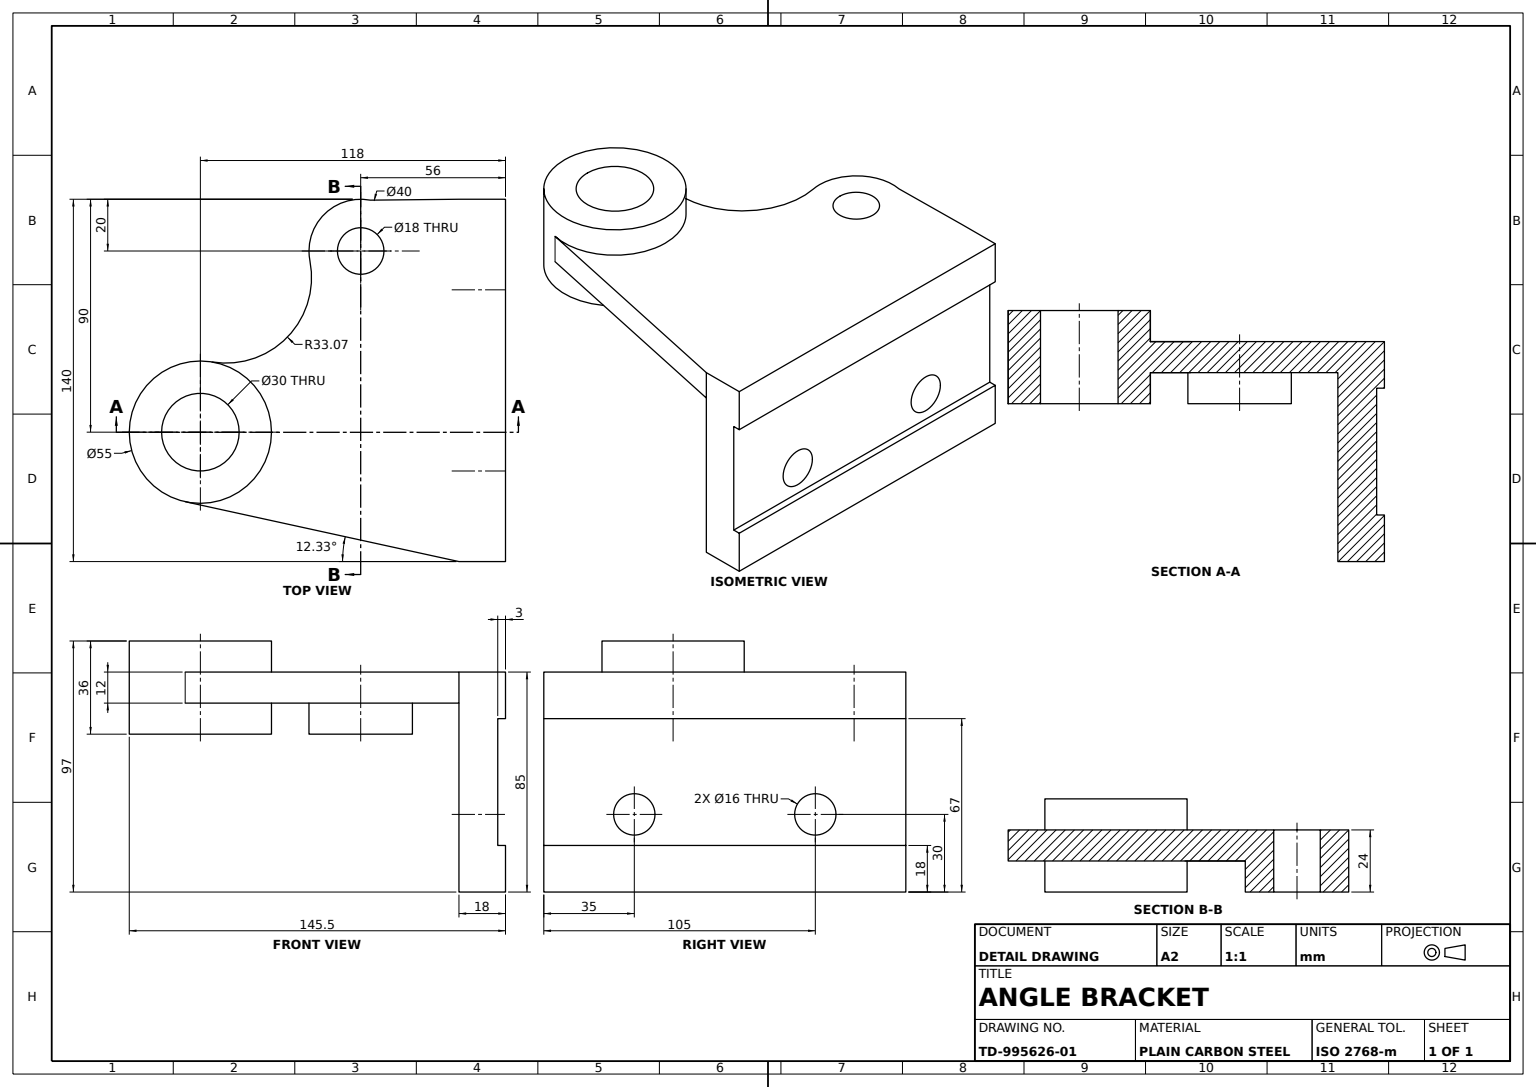
from build123d import *
from build123d.topology import SkipClean

# Parameters (mm, degrees)
BASE_PLATE_SKETCH_W             = 140
BASE_PLATE_SKETCH_H             = 85
BASE_PLATE_18MM_DEPTH           = 18
PLATE_PROFILE_CUT_SKETCH_W      = 3
PLATE_PROFILE_CUT_SKETCH_H      = 49
PLATE_PROFILE_CUT_DEPTH         = 140
NOTCH_16X16_SKETCH_R            = 8
NOTCH_16X16_DEPTH               = 140
SMALL_EYE_BOSS_40_SKETCH_R      = 20
SMALL_EYE_BOSS_40_DEPTH         = 12
LARGE_EYE_BOSS_55_SKETCH_R      = 27.5
LARGE_EYE_BOSS_55_DEPTH         = 12
EYE_LINK_WEB_DEPTH              = 12
LARGE_START                     = 12
LARGE_EYE_CAP_55_SKETCH_R       = 27.5
LARGE_EYE_CAP_55_DEPTH          = 12
LARGE_EYE_EXTENSION_55_SKETCH_R = 27.5
LARGE_EYE_EXTENSION_55_DEPTH    = 12
SMALL_EYE_EXTENSION_40_SKETCH_R = 20
SMALL_EYE_EXTENSION_40_DEPTH    = 12
LARGE_EYE_BORE_30_SKETCH_R      = 15
LARGE_EYE_BORE_30_DEPTH         = 36
SMALL_EYE_BORE_18_SKETCH_R      = 9
SMALL_EYE_BORE_18_DEPTH         = 24


with BuildPart() as part:
    # Base Plate Sketch → Base Plate 18mm (new body)
    with BuildSketch(Plane.XY):
        with Locations((70, -42.5)):
            Rectangle(BASE_PLATE_SKETCH_W, BASE_PLATE_SKETCH_H)
    extrude(amount=BASE_PLATE_18MM_DEPTH)

    # Plate Profile Cut Sketch → Plate Profile Cut (cut)
    with BuildSketch(Plane.ZY):
        with Locations((1.5, -42.5)):
            Rectangle(PLATE_PROFILE_CUT_SKETCH_W, PLATE_PROFILE_CUT_SKETCH_H)
    extrude(amount=-PLATE_PROFILE_CUT_DEPTH, mode=Mode.SUBTRACT)

    # Notch 16x16 Sketch → Notch 16x16 (cut)
    with BuildSketch(Plane.XY.offset(18)):
        with Locations((35, -55)):
            Circle(NOTCH_16X16_SKETCH_R)
        with Locations((105, -55)):
            Circle(NOTCH_16X16_SKETCH_R)
    extrude(amount=-NOTCH_16X16_DEPTH, mode=Mode.SUBTRACT)



with BuildPart() as body_2:
    # Small Eye Boss Ø40 Sketch → Small Eye Boss Ø40 (new body)
    with BuildSketch(Plane(origin=(0, 0, 0), x_dir=(1, 0, 0), z_dir=(0, 1, 0))):
        with Locations(Location((20, -56, 0), (0, 0, 270))):
            Circle(SMALL_EYE_BOSS_40_SKETCH_R)
    extrude(amount=-SMALL_EYE_BOSS_40_DEPTH)


with BuildPart() as body_3:
    # Large Eye Boss Ø55 Sketch → Large Eye Boss Ø55 (new body)
    with BuildSketch(Plane(origin=(0, 0, 0), x_dir=(1, 0, 0), z_dir=(0, 1, 0))):
        with Locations(Location((90, -118, 0), (0, 0, 270))):
            Circle(LARGE_EYE_BOSS_55_SKETCH_R)
    extrude(amount=-LARGE_EYE_BOSS_55_DEPTH)


with BuildPart() as part_1:
    add(part.part)

    add(body_2.part)  # Eye Link Web merges body 2

    add(body_3.part)  # Eye Link Web merges body 3
    # Eye Link Web Sketch → Eye Link Web (add)
    with BuildSketch(Plane(origin=(0, 0, 0), x_dir=(1, 0, 0), z_dir=(0, 1, 0))):
        with BuildLine():
            Line((0, -18), (0.353571949, -52.255956083))
            ThreePointArc((0.353571949, -52.255956083), (34.099175171, -41.815034032), (23.863156104, -75.623354069))
            ThreePointArc((23.863156104, -75.623354069), (53.284344418, -84.341805302), (62.872127171, -113.491284467))
            ThreePointArc((62.872127171, -113.491284467), (95.191280297, -90.994433743), (116.866088482, -123.870544241))
            Line((116.866088482, -123.870544241), (140, -18))
            Line((140, -18), (0, -18))
        make_face()
    extrude(amount=-EYE_LINK_WEB_DEPTH)

    # Large Eye Cap Ø55 Sketch → Large Eye Cap Ø55 (add)
    with BuildSketch(Plane(origin=(0, 0, 0), x_dir=(1, 0, 0), z_dir=(0, 1, 0)).offset(LARGE_START)):
        with Locations(Location((90, -118, 0), (0, 0, 270))):
            Circle(LARGE_EYE_CAP_55_SKETCH_R)
    extrude(amount=-LARGE_EYE_CAP_55_DEPTH)

    # Large Eye Extension Ø55 Sketch → Large Eye Extension Ø55 (add)
    with SkipClean():  # the faces are left unmerged after this step: merging them gives an invalid solid
        with BuildSketch(Plane.XZ.offset(12)):
            with Locations(Location((90, 118, 0), (0, 0, 90))):
                Circle(LARGE_EYE_EXTENSION_55_SKETCH_R)
        extrude(amount=LARGE_EYE_EXTENSION_55_DEPTH)

    # Small Eye Extension Ø40 Sketch → Small Eye Extension Ø40 (add)
    with SkipClean():  # the faces are left unmerged after this step: merging them gives an invalid solid
        with BuildSketch(Plane.XZ.offset(12)):
            with Locations(Location((20, 56, 0), (0, 0, 78.862872248))):
                Circle(SMALL_EYE_EXTENSION_40_SKETCH_R)
        extrude(amount=SMALL_EYE_EXTENSION_40_DEPTH)

    # Large Eye Bore Ø30 Sketch → Large Eye Bore Ø30 (cut)
    with SkipClean():  # the faces are left unmerged after this step: merging them gives an invalid solid
        with BuildSketch(Plane.XZ.offset(24)):
            with Locations(Location((90, 118, 0), (0, 0, 270))):
                Circle(LARGE_EYE_BORE_30_SKETCH_R)
        extrude(amount=-LARGE_EYE_BORE_30_DEPTH, mode=Mode.SUBTRACT)

    # Small Eye Bore Ø18 Sketch → Small Eye Bore Ø18 (cut)
    with SkipClean():  # the faces are left unmerged after this step: merging them gives an invalid solid
        with BuildSketch(Plane.XZ.offset(24)):
            with Locations(Location((20, 56, 0), (0, 0, 270))):
                Circle(SMALL_EYE_BORE_18_SKETCH_R)
        extrude(amount=-SMALL_EYE_BORE_18_DEPTH, mode=Mode.SUBTRACT)


solid = part_1.part
